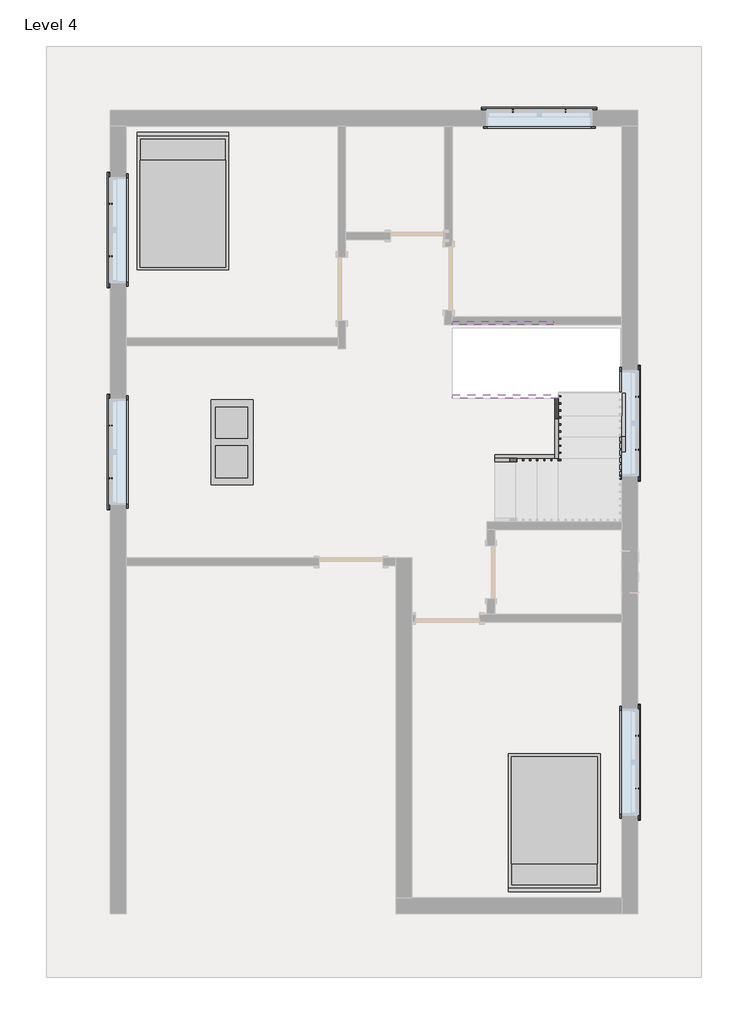
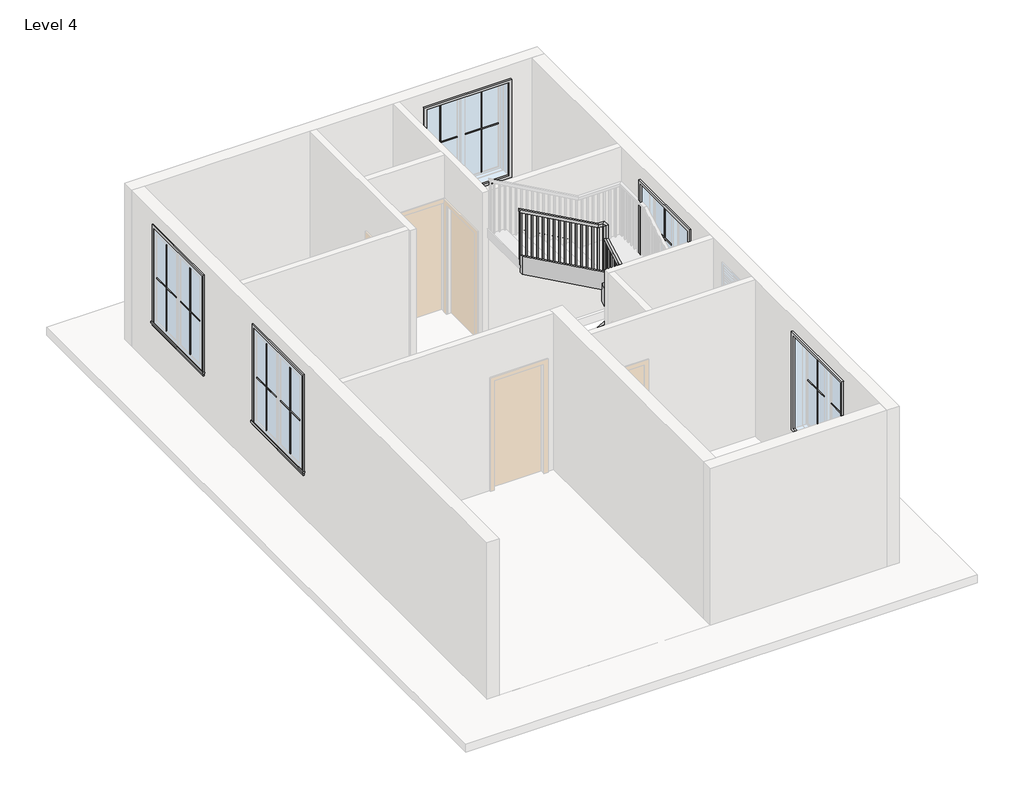
# One storey, part 2 of 2: 21 proxies, 6 members, 2 furniture elements, 1 railing.
"""IFC4 building model written with IfcOpenShell, lengths in millimetres."""

from ifc_helpers import new_model, si_unit, frame, origin, place, context, project, spatial, polyline, outline, extrude, faceted_brep, transform, mapped, element, save
from components import muntin_pattern_2x2_muntin_pattern_2x2_f6a80940, muntin_pattern_2x2_muntin_pattern_2x2_09b00a1c, trim_window_exterior_flat_with_sill_698ed857, trim_window_interior_flat_picture_frame_92551a5e, coffee_table_with_brass_mullions_11320_coffee_table_with_5962bef7, bed_17739_bed_17739_15c61121

model = new_model("IFC4")

# Units and contexts
model_context = context("Model", 3, world=origin())
ifc_project = project(units=[si_unit("LENGTHUNIT", "METRE", prefix="MILLI")], contexts=[model_context])

# Site, building, storey
site = spatial("IfcSite", under=ifc_project)
building = spatial("IfcBuilding", under=site)
storey = spatial("IfcBuildingStorey", under=building, Name="Level 4", Elevation=6400.8)

# Proxies
placement = place(None, origin())
muntin_pattern_2x2_muntin_pattern_2x2_shape = muntin_pattern_2x2_muntin_pattern_2x2_f6a80940(model_context)
element("IfcBuildingElementProxy", 1, Name="Muntin Pattern_2x2 : Muntin Pattern_2x2", ObjectType="Muntin Pattern_2x2 : Muntin Pattern_2x2", at=placement, inside=storey, context=model_context, shape_type="MappedRepresentation", body=[
    mapped(muntin_pattern_2x2_muntin_pattern_2x2_shape, transform((-4589.1575206, 441.8004493, 7385.05), x_axis=(0.0, 1.0, 0.0), y_axis=(-1.0, 0.0, 0.0), z_axis=(0.0, 0.0, 1.0))),
])
element("IfcBuildingElementProxy", 2, Name="Muntin Pattern_2x2 : Muntin Pattern_2x2", ObjectType="Muntin Pattern_2x2 : Muntin Pattern_2x2", at=placement, inside=storey, context=model_context, shape_type="MappedRepresentation", body=[
    mapped(muntin_pattern_2x2_muntin_pattern_2x2_shape, transform((-4589.1575206, 3632.6754493, 7385.05), x_axis=(0.0, 1.0, 0.0), y_axis=(-1.0, 0.0, 0.0), z_axis=(0.0, 0.0, 1.0))),
])
element("IfcBuildingElementProxy", 3, Name="Muntin Pattern_2x2 : Muntin Pattern_2x2", ObjectType="Muntin Pattern_2x2 : Muntin Pattern_2x2", at=placement, inside=storey, context=model_context, shape_type="MappedRepresentation", body=[
    mapped(muntin_pattern_2x2_muntin_pattern_2x2_shape, transform((1197.2799794, 5726.5879493, 7385.05), x_axis=(1.0, 0.0, 0.0), y_axis=(0.0, 1.0, 0.0), z_axis=(0.0, 0.0, 1.0))),
])
element("IfcBuildingElementProxy", 4, Name="Muntin Pattern_2x2 : Muntin Pattern_2x2", ObjectType="Muntin Pattern_2x2 : Muntin Pattern_2x2", at=placement, inside=storey, context=model_context, shape_type="MappedRepresentation", body=[
    mapped(muntin_pattern_2x2_muntin_pattern_2x2_shape, transform((2986.3924794, 1613.3754493, 7385.05), x_axis=(0.0, -1.0, 0.0), y_axis=(1.0, 0.0, 0.0), z_axis=(0.0, 0.0, 1.0))),
])
element("IfcBuildingElementProxy", 5, Name="Muntin Pattern_2x2 : Muntin Pattern_2x2", ObjectType="Muntin Pattern_2x2 : Muntin Pattern_2x2", at=placement, inside=storey, context=model_context, shape_type="MappedRepresentation", body=[
    mapped(muntin_pattern_2x2_muntin_pattern_2x2_shape, transform((2986.3924794, -3260.2495507, 7385.05), x_axis=(0.0, -1.0, 0.0), y_axis=(1.0, 0.0, 0.0), z_axis=(0.0, 0.0, 1.0))),
])
muntin_pattern_2x2_muntin_pattern_2x2_2_shape = muntin_pattern_2x2_muntin_pattern_2x2_09b00a1c(model_context)
element("IfcBuildingElementProxy", 6, Name="Muntin Pattern_2x2 : Muntin Pattern_2x2", ObjectType="Muntin Pattern_2x2 : Muntin Pattern_2x2", at=placement, inside=storey, context=model_context, shape_type="MappedRepresentation", body=[
    mapped(muntin_pattern_2x2_muntin_pattern_2x2_2_shape, transform((-4589.1575206, 1200.6254493, 7385.05), x_axis=(0.0, -1.0, 0.0), y_axis=(1.0, 0.0, 0.0), z_axis=(0.0, 0.0, 1.0))),
])
element("IfcBuildingElementProxy", 7, Name="Muntin Pattern_2x2 : Muntin Pattern_2x2", ObjectType="Muntin Pattern_2x2 : Muntin Pattern_2x2", at=placement, inside=storey, context=model_context, shape_type="MappedRepresentation", body=[
    mapped(muntin_pattern_2x2_muntin_pattern_2x2_2_shape, transform((-4589.1575206, 4391.5004493, 7385.05), x_axis=(0.0, -1.0, 0.0), y_axis=(1.0, 0.0, 0.0), z_axis=(0.0, 0.0, 1.0))),
])
element("IfcBuildingElementProxy", 8, Name="Muntin Pattern_2x2 : Muntin Pattern_2x2", ObjectType="Muntin Pattern_2x2 : Muntin Pattern_2x2", at=placement, inside=storey, context=model_context, shape_type="MappedRepresentation", body=[
    mapped(muntin_pattern_2x2_muntin_pattern_2x2_2_shape, transform((1956.1049794, 5726.5879493, 7385.05), x_axis=(-1.0, 0.0, 0.0), y_axis=(0.0, -1.0, 0.0), z_axis=(0.0, 0.0, 1.0))),
])
element("IfcBuildingElementProxy", 9, Name="Muntin Pattern_2x2 : Muntin Pattern_2x2", ObjectType="Muntin Pattern_2x2 : Muntin Pattern_2x2", at=placement, inside=storey, context=model_context, shape_type="MappedRepresentation", body=[
    mapped(muntin_pattern_2x2_muntin_pattern_2x2_2_shape, transform((2986.3924794, 854.5504493, 7385.05), x_axis=(0.0, 1.0, 0.0), y_axis=(-1.0, 0.0, 0.0), z_axis=(0.0, 0.0, 1.0))),
])
element("IfcBuildingElementProxy", 10, Name="Muntin Pattern_2x2 : Muntin Pattern_2x2", ObjectType="Muntin Pattern_2x2 : Muntin Pattern_2x2", at=placement, inside=storey, context=model_context, shape_type="MappedRepresentation", body=[
    mapped(muntin_pattern_2x2_muntin_pattern_2x2_2_shape, transform((2986.3924794, -4019.0745507, 7385.05), x_axis=(0.0, 1.0, 0.0), y_axis=(-1.0, 0.0, 0.0), z_axis=(0.0, 0.0, 1.0))),
])
trim_window_exterior_flat_with_sill_shape = trim_window_exterior_flat_with_sill_698ed857(model_context)
element("IfcBuildingElementProxy", 11, Name="Trim-Window-Exterior-Flat : with Sill", ObjectType="Trim-Window-Exterior-Flat : with Sill", at=placement, inside=storey, context=model_context, shape_type="MappedRepresentation", body=[
    mapped(trim_window_exterior_flat_with_sill_shape, transform((-4598.6825206, 821.2129493, 9144.0), x_axis=(0.0, -1.0, 0.0), y_axis=(0.0, 0.0, 1.0), z_axis=(-1.0, 0.0, 0.0))),
])
element("IfcBuildingElementProxy", 12, Name="Trim-Window-Exterior-Flat : with Sill", ObjectType="Trim-Window-Exterior-Flat : with Sill", at=placement, inside=storey, context=model_context, shape_type="MappedRepresentation", body=[
    mapped(trim_window_exterior_flat_with_sill_shape, transform((-4598.6825206, 4012.0879493, 9144.0), x_axis=(0.0, -1.0, 0.0), y_axis=(0.0, 0.0, 1.0), z_axis=(-1.0, 0.0, 0.0))),
])
element("IfcBuildingElementProxy", 13, Name="Trim-Window-Exterior-Flat : with Sill", ObjectType="Trim-Window-Exterior-Flat : with Sill", at=placement, inside=storey, context=model_context, shape_type="MappedRepresentation", body=[
    mapped(trim_window_exterior_flat_with_sill_shape, transform((1576.6924794, 5736.1129493, 9144.0), x_axis=(-1.0, 0.0, 0.0), y_axis=(0.0, 0.0, 1.0), z_axis=(0.0, 1.0, 0.0))),
])
element("IfcBuildingElementProxy", 14, Name="Trim-Window-Exterior-Flat : with Sill", ObjectType="Trim-Window-Exterior-Flat : with Sill", at=placement, inside=storey, context=model_context, shape_type="MappedRepresentation", body=[
    mapped(trim_window_exterior_flat_with_sill_shape, transform((2995.9174794, 1233.9629493, 9144.0), x_axis=(0.0, 1.0, 0.0), y_axis=(0.0, 0.0, 1.0), z_axis=(1.0, 0.0, 0.0))),
])
element("IfcBuildingElementProxy", 15, Name="Trim-Window-Exterior-Flat : with Sill", ObjectType="Trim-Window-Exterior-Flat : with Sill", at=placement, inside=storey, context=model_context, shape_type="MappedRepresentation", body=[
    mapped(trim_window_exterior_flat_with_sill_shape, transform((2995.9174794, -3639.6620507, 9144.0), x_axis=(0.0, 1.0, 0.0), y_axis=(0.0, 0.0, 1.0), z_axis=(1.0, 0.0, 0.0))),
])
trim_window_interior_flat_picture_frame_shape = trim_window_interior_flat_picture_frame_92551a5e(model_context)
element("IfcBuildingElementProxy", 16, Name="Trim-Window-Interior-Flat : Picture Frame", ObjectType="Trim-Window-Interior-Flat : Picture Frame", at=placement, inside=storey, context=model_context, shape_type="MappedRepresentation", body=[
    mapped(trim_window_interior_flat_picture_frame_shape, transform((-4370.0825206, 821.2129493, 9144.0), x_axis=(0.0, 1.0, 0.0), y_axis=(0.0, 0.0, 1.0), z_axis=(1.0, 0.0, 0.0))),
])
element("IfcBuildingElementProxy", 17, Name="Trim-Window-Interior-Flat : Picture Frame", ObjectType="Trim-Window-Interior-Flat : Picture Frame", at=placement, inside=storey, context=model_context, shape_type="MappedRepresentation", body=[
    mapped(trim_window_interior_flat_picture_frame_shape, transform((-4370.0825206, 4012.0879493, 9144.0), x_axis=(0.0, 1.0, 0.0), y_axis=(0.0, 0.0, 1.0), z_axis=(1.0, 0.0, 0.0))),
])
element("IfcBuildingElementProxy", 18, Name="Trim-Window-Interior-Flat : Picture Frame", ObjectType="Trim-Window-Interior-Flat : Picture Frame", at=placement, inside=storey, context=model_context, shape_type="MappedRepresentation", body=[
    mapped(trim_window_interior_flat_picture_frame_shape, transform((1576.6924794, 5507.5129493, 9144.0), x_axis=(1.0, 0.0, 0.0), y_axis=(0.0, 0.0, 1.0), z_axis=(0.0, -1.0, 0.0))),
])
element("IfcBuildingElementProxy", 19, Name="Trim-Window-Interior-Flat : Picture Frame", ObjectType="Trim-Window-Interior-Flat : Picture Frame", at=placement, inside=storey, context=model_context, shape_type="MappedRepresentation", body=[
    mapped(trim_window_interior_flat_picture_frame_shape, transform((2767.3174794, 1233.9629493, 9144.0), x_axis=(0.0, -1.0, 0.0), y_axis=(0.0, 0.0, 1.0), z_axis=(-1.0, 0.0, 0.0))),
])
element("IfcBuildingElementProxy", 20, Name="Trim-Window-Interior-Flat : Picture Frame", ObjectType="Trim-Window-Interior-Flat : Picture Frame", at=placement, inside=storey, context=model_context, shape_type="MappedRepresentation", body=[
    mapped(trim_window_interior_flat_picture_frame_shape, transform((2767.3174794, -3639.6620507, 9144.0), x_axis=(0.0, -1.0, 0.0), y_axis=(0.0, 0.0, 1.0), z_axis=(-1.0, 0.0, 0.0))),
])
coffee_table_with_brass_mullions_11320_coffee_table_with_shape = coffee_table_with_brass_mullions_11320_coffee_table_with_5962bef7(model_context)
element("IfcBuildingElementProxy", 21, Name="coffee_table_with_brass_mullions_11320 : coffee_table_with_brass_mullions_11320", ObjectType="coffee_table_with_brass_mullions_11320 : coffee_table_with_brass_mullions_11320", at=placement, inside=storey, context=model_context, shape_type="MappedRepresentation", body=[
    mapped(coffee_table_with_brass_mullions_11320_coffee_table_with_shape, transform((-2412.0418112, 1596.9678033, 6400.8), x_axis=(0.0, 1.0, 0.0), y_axis=(-1.0, 0.0, 0.0), z_axis=(0.0, 0.0, 1.0))),
])

# Furniture
bed_17739_bed_17739_shape = bed_17739_bed_17739_15c61121(model_context)
element("IfcFurniture", 22, ObjectType="Bed_17739 : Bed_17739", at=placement, inside=storey, context=model_context, shape_type="MappedRepresentation", body=[
    mapped(bed_17739_bed_17739_shape, transform((-3550.9325206, 4402.6129493, 6400.8), x_axis=(1.0, 0.0, 0.0), y_axis=(0.0, 1.0, 0.0), z_axis=(0.0, 0.0, 1.0))),
])
element("IfcFurniture", 23, ObjectType="Bed_17739 : Bed_17739", at=placement, inside=storey, context=model_context, shape_type="MappedRepresentation", body=[
    mapped(bed_17739_bed_17739_shape, transform((1795.7674794, -4487.3870507, 6400.8), x_axis=(-1.0, 0.0, 0.0), y_axis=(0.0, -1.0, 0.0), z_axis=(0.0, 0.0, 1.0))),
])

# Members
element("IfcMember", 24, ObjectType="Stringer - 2\" Width", at=placement, inside=storey, context=model_context, shape_type="SweptSolid", body=[
    extrude(outline(polyline([(6608.3983948, 938.5174794), (6400.8, 938.5174794), (6400.8, 1192.4619822), (6739.4974984, 1802.1174794), (7088.1761726, 1802.1174794), (6608.3983948, 938.5174794)])), frame((0.0, 732.3129493, 0.0), z_axis=(0.0, 1.0, 0.0), x_axis=(0.0, 0.0, 1.0)), (0.0, 0.0, 1.0), 50.8),
])
element("IfcMember", 25, ObjectType="Stringer - 2\" Width", at=placement, inside=storey, context=model_context, shape_type="SweptSolid", body=[
    extrude(outline(polyline([(732.3129493, 6937.053054), (732.3129493, 7285.7317281), (1595.9129493, 7765.5095059), (1595.9129493, 7416.8308318), (732.3129493, 6937.053054)])), frame((1802.1174794, 0.0, 0.0), z_axis=(1.0, 0.0, 0.0), x_axis=(0.0, 1.0, 0.0)), (0.0, 0.0, 1.0), 50.8),
])
element("IfcMember", 26, ObjectType="Stringer - 2\" Width", at=placement, inside=storey, context=model_context, shape_type="SweptSolid", body=[
    extrude(outline(polyline([(7614.3863873, 1852.9174794), (7963.0650614, 1852.9174794), (8809.7317281, 328.9174794), (8461.053054, 328.9174794), (7614.3863873, 1852.9174794)])), frame((0.0, 1595.9129493, 0.0), z_axis=(0.0, 1.0, 0.0), x_axis=(0.0, 0.0, 1.0)), (0.0, 0.0, 1.0), 50.8),
])
element("IfcMember", 27, ObjectType="Stringer - 2\" Width", at=placement, inside=storey, context=model_context, shape_type="SweptSolid", body=[
    extrude(outline(polyline([(6608.3983948, 938.5174794), (6400.8, 938.5174794), (6400.8, 1192.4619822), (6777.7317281, 1870.9390928), (6777.7317281, 1243.3174794), (6608.3983948, 938.5174794)])), frame((0.0, -232.8870507, 0.0), z_axis=(0.0, 1.0, 0.0), x_axis=(0.0, 0.0, 1.0)), (0.0, 0.0, 1.0), 50.8),
])
element("IfcMember", 28, ObjectType="Stringer - 2\" Width", at=placement, inside=storey, context=model_context, shape_type="SweptSolid", body=[
    extrude(outline(polyline([(714.2913359, 7275.7197207), (1037.1129493, 7455.0650614), (1664.7345627, 7455.0650614), (1341.9129493, 7275.7197207), (714.2913359, 7275.7197207)])), frame((2767.3174794, 0.0, 0.0), z_axis=(1.0, 0.0, 0.0), x_axis=(0.0, 1.0, 0.0)), (0.0, 0.0, 1.0), 50.8),
])
element("IfcMember", 29, ObjectType="Stringer - 2\" Width", at=placement, inside=storey, context=model_context, shape_type="SweptSolid", body=[
    extrude(outline(polyline([(8002.4419429, 1782.0390928), (8809.7317281, 328.9174794), (8461.053054, 328.9174794), (8002.4419429, 1154.4174794), (8002.4419429, 1782.0390928)])), frame((0.0, 2650.0129493, 0.0), z_axis=(0.0, 1.0, 0.0), x_axis=(0.0, 0.0, 1.0)), (0.0, 0.0, 1.0), 50.8),
])

# Railing
element("IfcRailing", 30, ObjectType="Handrail - Rectangular", at=placement, inside=storey, context=model_context, shape_type="SolidModel", body=[
    faceted_brep([(938.5174794, 732.3129493, 7484.5333333), (938.5174794, 732.3129493, 7426.420221), (938.5174794, 681.5129493, 7426.420221), (938.5174794, 681.5129493, 7484.5333333), (1776.7174794, 732.3129493, 7950.2), (1827.5174794, 732.3129493, 7920.3091099), (1827.5174794, 681.5129493, 7920.3091099), (1776.7174794, 681.5129493, 7950.2), (1776.7174794, 732.3129493, 8204.2), (1827.5174794, 732.3129493, 8153.4), (1827.5174794, 681.5129493, 8153.4), (1776.7174794, 681.5129493, 8204.2), (1852.9174794, 732.3129493, 8204.2), (1852.9174794, 732.3129493, 8153.4), (1903.7174794, 681.5129493, 8153.4), (1903.7174794, 681.5129493, 8204.2), (1852.9174794, 808.5129493, 8204.2), (1852.9174794, 821.6765516, 8153.4), (1903.7174794, 821.6765516, 8153.4), (1903.7174794, 808.5129493, 8204.2), (1852.9174794, 1570.5129493, 8627.5333333), (1852.9174794, 1621.3129493, 8597.6424432), (1903.7174794, 1621.3129493, 8597.6424432), (1903.7174794, 1570.5129493, 8627.5333333), (1852.9174794, 1570.5129493, 8881.5333333), (1852.9174794, 1621.3129493, 8830.7333333), (1903.7174794, 1621.3129493, 8830.7333333), (1903.7174794, 1570.5129493, 8881.5333333), (1852.9174794, 1646.7129493, 8881.5333333), (1852.9174794, 1646.7129493, 8830.7333333), (1903.7174794, 1697.5129493, 8830.7333333), (1903.7174794, 1697.5129493, 8881.5333333), (1776.7174794, 1646.7129493, 8881.5333333), (1763.5538772, 1646.7129493, 8830.7333333), (1763.5538772, 1697.5129493, 8830.7333333), (1776.7174794, 1697.5129493, 8881.5333333), (328.9174794, 1646.7129493, 9685.8666667), (328.9174794, 1697.5129493, 9685.8666667), (328.9174794, 1697.5129493, 9627.7535543), (328.9174794, 1646.7129493, 9627.7535543)], [[[0, 1, 2, 3]], [[1, 0, 4, 5]], [[2, 1, 5, 6]], [[3, 2, 6, 7]], [[0, 3, 7, 4]], [[5, 4, 8, 9]], [[6, 5, 9, 10]], [[7, 6, 10, 11]], [[4, 7, 11, 8]], [[9, 8, 12, 13]], [[10, 9, 13, 14]], [[11, 10, 14, 15]], [[8, 11, 15, 12]], [[13, 12, 16, 17]], [[14, 13, 17, 18]], [[15, 14, 18, 19]], [[12, 15, 19, 16]], [[17, 16, 20, 21]], [[18, 17, 21, 22]], [[19, 18, 22, 23]], [[16, 19, 23, 20]], [[21, 20, 24, 25]], [[22, 21, 25, 26]], [[23, 22, 26, 27]], [[20, 23, 27, 24]], [[25, 24, 28, 29]], [[26, 25, 29, 30]], [[27, 26, 30, 31]], [[24, 27, 31, 28]], [[29, 28, 32, 33]], [[30, 29, 33, 34]], [[31, 30, 34, 35]], [[28, 31, 35, 32]], [[36, 37, 38, 39]], [[33, 32, 36, 39]], [[34, 33, 39, 38]], [[35, 34, 38, 37]], [[32, 35, 37, 36]]]),
    extrude(outline(polyline([(9618.9341099, 344.7924794), (8602.1333333, 344.7924794), (8602.1333333, 363.8424794), (9608.3507765, 363.8424794), (9618.9341099, 344.7924794)])), frame((0.0, 1662.5879493, 0.0), z_axis=(0.0, 1.0, 0.0), x_axis=(0.0, 0.0, 1.0)), (0.0, 0.0, 1.0), 19.05),
    extrude(outline(polyline([(9562.4896654, 446.3924794), (8602.1333333, 446.3924794), (8602.1333333, 465.4424794), (9551.9063321, 465.4424794), (9562.4896654, 446.3924794)])), frame((0.0, 1662.5879493, 0.0), z_axis=(0.0, 1.0, 0.0), x_axis=(0.0, 0.0, 1.0)), (0.0, 0.0, 1.0), 19.05),
    extrude(outline(polyline([(9506.045221, 547.9924794), (8602.1333333, 547.9924794), (8602.1333333, 567.0424794), (9495.4618876, 567.0424794), (9506.045221, 547.9924794)])), frame((0.0, 1662.5879493, 0.0), z_axis=(0.0, 1.0, 0.0), x_axis=(0.0, 0.0, 1.0)), (0.0, 0.0, 1.0), 19.05),
    extrude(outline(polyline([(9449.6007765, 649.5924794), (8432.8, 649.5924794), (8432.8, 668.6424794), (9439.0174432, 668.6424794), (9449.6007765, 649.5924794)])), frame((0.0, 1662.5879493, 0.0), z_axis=(0.0, 1.0, 0.0), x_axis=(0.0, 0.0, 1.0)), (0.0, 0.0, 1.0), 19.05),
    extrude(outline(polyline([(9393.1563321, 751.1924794), (8432.8, 751.1924794), (8432.8, 770.2424794), (9382.5729988, 770.2424794), (9393.1563321, 751.1924794)])), frame((0.0, 1662.5879493, 0.0), z_axis=(0.0, 1.0, 0.0), x_axis=(0.0, 0.0, 1.0)), (0.0, 0.0, 1.0), 19.05),
    extrude(outline(polyline([(9336.7118876, 852.7924794), (8432.8, 852.7924794), (8432.8, 871.8424794), (9326.1285543, 871.8424794), (9336.7118876, 852.7924794)])), frame((0.0, 1662.5879493, 0.0), z_axis=(0.0, 1.0, 0.0), x_axis=(0.0, 0.0, 1.0)), (0.0, 0.0, 1.0), 19.05),
    extrude(outline(polyline([(9280.2674432, 954.3924794), (8263.4666667, 954.3924794), (8263.4666667, 973.4424794), (9269.6841099, 973.4424794), (9280.2674432, 954.3924794)])), frame((0.0, 1662.5879493, 0.0), z_axis=(0.0, 1.0, 0.0), x_axis=(0.0, 0.0, 1.0)), (0.0, 0.0, 1.0), 19.05),
    extrude(outline(polyline([(9223.8229988, 1055.9924794), (8263.4666667, 1055.9924794), (8263.4666667, 1075.0424794), (9213.2396654, 1075.0424794), (9223.8229988, 1055.9924794)])), frame((0.0, 1662.5879493, 0.0), z_axis=(0.0, 1.0, 0.0), x_axis=(0.0, 0.0, 1.0)), (0.0, 0.0, 1.0), 19.05),
    extrude(outline(polyline([(9167.3785543, 1157.5924794), (8263.4666667, 1157.5924794), (8263.4666667, 1176.6424794), (9156.795221, 1176.6424794), (9167.3785543, 1157.5924794)])), frame((0.0, 1662.5879493, 0.0), z_axis=(0.0, 1.0, 0.0), x_axis=(0.0, 0.0, 1.0)), (0.0, 0.0, 1.0), 19.05),
    extrude(outline(polyline([(9110.9341099, 1259.1924794), (8094.1333333, 1259.1924794), (8094.1333333, 1278.2424794), (9100.3507765, 1278.2424794), (9110.9341099, 1259.1924794)])), frame((0.0, 1662.5879493, 0.0), z_axis=(0.0, 1.0, 0.0), x_axis=(0.0, 0.0, 1.0)), (0.0, 0.0, 1.0), 19.05),
    extrude(outline(polyline([(9054.4896654, 1360.7924794), (8094.1333333, 1360.7924794), (8094.1333333, 1379.8424794), (9043.9063321, 1379.8424794), (9054.4896654, 1360.7924794)])), frame((0.0, 1662.5879493, 0.0), z_axis=(0.0, 1.0, 0.0), x_axis=(0.0, 0.0, 1.0)), (0.0, 0.0, 1.0), 19.05),
    extrude(outline(polyline([(8998.045221, 1462.3924794), (8094.1333333, 1462.3924794), (8094.1333333, 1481.4424794), (8987.4618876, 1481.4424794), (8998.045221, 1462.3924794)])), frame((0.0, 1662.5879493, 0.0), z_axis=(0.0, 1.0, 0.0), x_axis=(0.0, 0.0, 1.0)), (0.0, 0.0, 1.0), 19.05),
    extrude(outline(polyline([(8941.6007765, 1563.9924794), (7924.8, 1563.9924794), (7924.8, 1583.0424794), (8931.0174432, 1583.0424794), (8941.6007765, 1563.9924794)])), frame((0.0, 1662.5879493, 0.0), z_axis=(0.0, 1.0, 0.0), x_axis=(0.0, 0.0, 1.0)), (0.0, 0.0, 1.0), 19.05),
    extrude(outline(polyline([(8885.1563321, 1665.5924794), (7924.8, 1665.5924794), (7924.8, 1684.6424794), (8874.5729988, 1684.6424794), (8885.1563321, 1665.5924794)])), frame((0.0, 1662.5879493, 0.0), z_axis=(0.0, 1.0, 0.0), x_axis=(0.0, 0.0, 1.0)), (0.0, 0.0, 1.0), 19.05),
    extrude(outline(polyline([(8828.7118876, 1767.1924794), (7924.8, 1767.1924794), (7924.8, 1786.2424794), (8818.1285543, 1786.2424794), (8828.7118876, 1767.1924794)])), frame((0.0, 1662.5879493, 0.0), z_axis=(0.0, 1.0, 0.0), x_axis=(0.0, 0.0, 1.0)), (0.0, 0.0, 1.0), 19.05),
    extrude(outline(polyline([(1868.7924794, 1611.7879493), (1868.7924794, 1630.8379493), (1887.8424794, 1630.8379493), (1887.8424794, 1611.7879493), (1868.7924794, 1611.7879493)])), frame((0.0, 0.0, 7586.1333333), z_axis=(0.0, 0.0, 1.0), x_axis=(1.0, 0.0, 0.0)), (0.0, 0.0, 1.0), 1244.6),
    extrude(outline(polyline([(1529.2379493, 8546.4896654), (1529.2379493, 7586.1333333), (1510.1879493, 7586.1333333), (1510.1879493, 8535.9063321), (1529.2379493, 8546.4896654)])), frame((1868.7924794, 0.0, 0.0), z_axis=(1.0, 0.0, 0.0), x_axis=(0.0, 1.0, 0.0)), (0.0, 0.0, 1.0), 19.05),
    extrude(outline(polyline([(1427.6379493, 8490.045221), (1427.6379493, 7586.1333333), (1408.5879493, 7586.1333333), (1408.5879493, 8479.4618876), (1427.6379493, 8490.045221)])), frame((1868.7924794, 0.0, 0.0), z_axis=(1.0, 0.0, 0.0), x_axis=(0.0, 1.0, 0.0)), (0.0, 0.0, 1.0), 19.05),
    extrude(outline(polyline([(1326.0379493, 8433.6007765), (1326.0379493, 7416.8), (1306.9879493, 7416.8), (1306.9879493, 8423.0174432), (1326.0379493, 8433.6007765)])), frame((1868.7924794, 0.0, 0.0), z_axis=(1.0, 0.0, 0.0), x_axis=(0.0, 1.0, 0.0)), (0.0, 0.0, 1.0), 19.05),
    extrude(outline(polyline([(1224.4379493, 8377.1563321), (1224.4379493, 7416.8), (1205.3879493, 7416.8), (1205.3879493, 8366.5729988), (1224.4379493, 8377.1563321)])), frame((1868.7924794, 0.0, 0.0), z_axis=(1.0, 0.0, 0.0), x_axis=(0.0, 1.0, 0.0)), (0.0, 0.0, 1.0), 19.05),
    extrude(outline(polyline([(1122.8379493, 8320.7118876), (1122.8379493, 7416.8), (1103.7879493, 7416.8), (1103.7879493, 8310.1285543), (1122.8379493, 8320.7118876)])), frame((1868.7924794, 0.0, 0.0), z_axis=(1.0, 0.0, 0.0), x_axis=(0.0, 1.0, 0.0)), (0.0, 0.0, 1.0), 19.05),
    extrude(outline(polyline([(1021.2379493, 8264.2674432), (1021.2379493, 7247.4666667), (1002.1879493, 7247.4666667), (1002.1879493, 8253.6841099), (1021.2379493, 8264.2674432)])), frame((1868.7924794, 0.0, 0.0), z_axis=(1.0, 0.0, 0.0), x_axis=(0.0, 1.0, 0.0)), (0.0, 0.0, 1.0), 19.05),
    extrude(outline(polyline([(919.6379493, 8207.8229988), (919.6379493, 7247.4666667), (900.5879493, 7247.4666667), (900.5879493, 8197.2396654), (919.6379493, 8207.8229988)])), frame((1868.7924794, 0.0, 0.0), z_axis=(1.0, 0.0, 0.0), x_axis=(0.0, 1.0, 0.0)), (0.0, 0.0, 1.0), 19.05),
    extrude(outline(polyline([(818.0379493, 8151.3785543), (818.0379493, 7247.4666667), (798.9879493, 7247.4666667), (798.9879493, 8140.795221), (818.0379493, 8151.3785543)])), frame((1868.7924794, 0.0, 0.0), z_axis=(1.0, 0.0, 0.0), x_axis=(0.0, 1.0, 0.0)), (0.0, 0.0, 1.0), 19.05),
    extrude(outline(polyline([(1843.3924794, 716.4379493), (1862.4424794, 716.4379493), (1862.4424794, 697.3879493), (1843.3924794, 697.3879493), (1843.3924794, 716.4379493)])), frame((0.0, 0.0, 7078.1333333), z_axis=(0.0, 0.0, 1.0), x_axis=(1.0, 0.0, 0.0)), (0.0, 0.0, 1.0), 1075.2666667),
    extrude(outline(polyline([(7872.6841099, 1741.7924794), (6908.8, 1741.7924794), (6908.8, 1760.8424794), (7883.2674432, 1760.8424794), (7872.6841099, 1741.7924794)])), frame((0.0, 697.3879493, 0.0), z_axis=(0.0, 1.0, 0.0), x_axis=(0.0, 0.0, 1.0)), (0.0, 0.0, 1.0), 19.05),
    extrude(outline(polyline([(7816.2396654, 1640.1924794), (6908.8, 1640.1924794), (6908.8, 1659.2424794), (7826.8229988, 1659.2424794), (7816.2396654, 1640.1924794)])), frame((0.0, 697.3879493, 0.0), z_axis=(0.0, 1.0, 0.0), x_axis=(0.0, 0.0, 1.0)), (0.0, 0.0, 1.0), 19.05),
    extrude(outline(polyline([(7759.795221, 1538.5924794), (6908.8, 1538.5924794), (6908.8, 1557.6424794), (7770.3785543, 1557.6424794), (7759.795221, 1538.5924794)])), frame((0.0, 697.3879493, 0.0), z_axis=(0.0, 1.0, 0.0), x_axis=(0.0, 0.0, 1.0)), (0.0, 0.0, 1.0), 19.05),
    extrude(outline(polyline([(7703.3507765, 1436.9924794), (6739.4666667, 1436.9924794), (6739.4666667, 1456.0424794), (7713.9341099, 1456.0424794), (7703.3507765, 1436.9924794)])), frame((0.0, 697.3879493, 0.0), z_axis=(0.0, 1.0, 0.0), x_axis=(0.0, 0.0, 1.0)), (0.0, 0.0, 1.0), 19.05),
    extrude(outline(polyline([(7646.9063321, 1335.3924794), (6739.4666667, 1335.3924794), (6739.4666667, 1354.4424794), (7657.4896654, 1354.4424794), (7646.9063321, 1335.3924794)])), frame((0.0, 697.3879493, 0.0), z_axis=(0.0, 1.0, 0.0), x_axis=(0.0, 0.0, 1.0)), (0.0, 0.0, 1.0), 19.05),
    extrude(outline(polyline([(7590.4618876, 1233.7924794), (6739.4666667, 1233.7924794), (6739.4666667, 1252.8424794), (7601.045221, 1252.8424794), (7590.4618876, 1233.7924794)])), frame((0.0, 697.3879493, 0.0), z_axis=(0.0, 1.0, 0.0), x_axis=(0.0, 0.0, 1.0)), (0.0, 0.0, 1.0), 19.05),
    extrude(outline(polyline([(7534.0174432, 1132.1924794), (6570.1333333, 1132.1924794), (6570.1333333, 1151.2424794), (7544.6007765, 1151.2424794), (7534.0174432, 1132.1924794)])), frame((0.0, 697.3879493, 0.0), z_axis=(0.0, 1.0, 0.0), x_axis=(0.0, 0.0, 1.0)), (0.0, 0.0, 1.0), 19.05),
    extrude(outline(polyline([(7477.5729988, 1030.5924794), (6570.1333333, 1030.5924794), (6570.1333333, 1049.6424794), (7488.1563321, 1049.6424794), (7477.5729988, 1030.5924794)])), frame((0.0, 697.3879493, 0.0), z_axis=(0.0, 1.0, 0.0), x_axis=(0.0, 0.0, 1.0)), (0.0, 0.0, 1.0), 19.05),
    extrude(outline(polyline([(1868.7924794, 1662.5879493), (1868.7924794, 1681.6379493), (1887.8424794, 1681.6379493), (1887.8424794, 1662.5879493), (1868.7924794, 1662.5879493)])), frame((0.0, 0.0, 7755.4666667), z_axis=(0.0, 0.0, 1.0), x_axis=(1.0, 0.0, 0.0)), (0.0, 0.0, 1.0), 1075.2666667),
    extrude(outline(polyline([(1868.7924794, 716.4379493), (1887.8424794, 716.4379493), (1887.8424794, 697.3879493), (1868.7924794, 697.3879493), (1868.7924794, 716.4379493)])), frame((0.0, 0.0, 7078.1333333), z_axis=(0.0, 0.0, 1.0), x_axis=(1.0, 0.0, 0.0)), (0.0, 0.0, 1.0), 1075.2666667),
    extrude(outline(polyline([(9627.7535543, 328.9174794), (8602.1333333, 328.9174794), (8602.1333333, 347.9674794), (9617.170221, 347.9674794), (9627.7535543, 328.9174794)])), frame((0.0, 1662.5879493, 0.0), z_axis=(0.0, 1.0, 0.0), x_axis=(0.0, 0.0, 1.0)), (0.0, 0.0, 1.0), 19.05),
    extrude(outline(polyline([(7426.420221, 938.5174794), (6570.1333333, 938.5174794), (6570.1333333, 957.5674794), (7437.0035543, 957.5674794), (7426.420221, 938.5174794)])), frame((0.0, 697.3879493, 0.0), z_axis=(0.0, 1.0, 0.0), x_axis=(0.0, 0.0, 1.0)), (0.0, 0.0, 1.0), 19.05),
])

save(model, "model.ifc")

# Revit data of these elements
# Type "Muntin Pattern_2x2 : Muntin Pattern_2x2"
#   Width [instance default] = 4' - 0"
#   Thickness = 0' - 0 1/2"
#   Height [instance default] = 4' - 0"
#   Distance = 0' - 0 3/4"
#   Interior Material [instance default] = none
#   Exterior Material [instance default] = none
#   Default Elevation = 0
# Type "Trim-Window-Exterior-Flat : with Sill"
#   Trim Width = 0' - 2 1/4"
#   Trim Thickness_Picture Frame = 0' - 1 1/4"
#   Trim Thickness_with Sill = 0' - 0 3/4"
#   Sill Thickness = 0' - 1 1/4"
#   Opening Width [instance default] = 2' - 0"
#   Opening Height [instance default] = 3' - 0"
#   Default Elevation = 4' - 0"
#   Sill = yes
#   Picture Frame = no
#   Trim Material [instance default] = none
# Type "Trim-Window-Interior-Flat : Picture Frame"
#   Trim Thickness_Picture Frame = 0' - 1 1/4"
#   Trim Width = 0' - 2 1/4"
#   Trim Thickness_with Sill = 0' - 0 3/4"
#   Sill Thickness = 0' - 1 1/4"
#   Opening Width [instance default] = 2' - 0"
#   Opening Height [instance default] = 3' - 0"
#   Default Elevation = 4' - 0"
#   Sill = no
#   Picture Frame = yes
#   Trim Material [instance default] = none
# Type "coffee_table_with_brass_mullions_11320 : coffee_table_with_brass_mullions_11320"
#   Default Elevation = 0
# Type "Bed_17739 : Bed_17739"
#   Default Elevation = 0
# Type "Handrail - Rectangular"
#   Assembly Code = "C2010400"
#   built-in parameter 1008612 = 0.0416667 (stored number, unit not read)
#   built-in parameter 1008611 = 0.0416667 (stored number, unit not read)
#   built-in parameter 1008609 = 0.333333 (stored number, unit not read)
#   built-in parameter 1008604 = 0.166667 (stored number, unit not read)
#   built-in parameter 1008603 = 0.166667 (stored number, unit not read)
#   Railing Height = 3' - 0"
#   built-in parameter 1008630 = 2
#   built-in parameter 1008610 = 2
#   built-in parameter 1008618 = Baluster - Square : 3/4"
# Elements 1, 2, 3, 4, 5, 6, 7, 8, 9, 10 (IfcBuildingElementProxy, "Muntin Pattern_2x2 : Muntin Pattern_2x2")
#   Width = 2' - 0 5/8"
#   Height = 5' - 6 1/2"
#   Interior Material = Wood - Stained
#   Exterior Material = Clad - White
#   Phase Created = New Construction
#   Materials on its faces: "Clad - White", "Wood - Stained"
# Elements 11, 12, 13, 14, 15 (IfcBuildingElementProxy, "Trim-Window-Exterior-Flat : with Sill")
#   Opening Width = 5' - 0"
#   Opening Height = 6' - 0"
#   Trim Material = Clad - White
#   Phase Created = New Construction
#   Materials on its faces: "Clad - White"
# Elements 16, 17, 18, 19, 20 (IfcBuildingElementProxy, "Trim-Window-Interior-Flat : Picture Frame")
#   Opening Width = 5' - 0"
#   Opening Height = 6' - 0"
#   Trim Material = Wood - Stained
#   Phase Created = New Construction
#   Materials on its faces: "Wood - Stained"
# Element 21 (IfcBuildingElementProxy, "coffee_table_with_brass_mullions_11320 : coffee_table_with_brass_mullions_11320")
#   Phase Created = New Construction
#   Materials on its faces: "Default Wall", "TABLE", "Glass", "Default"
# Elements 22, 23 (IfcFurniture, "Bed_17739 : Bed_17739")
#   Phase Created = New Construction
#   Materials on its faces: "legs", "sheets", "bed frame", "Blanket"
# Elements 24, 25, 26, 27, 28, 29 (IfcMember, "Stringer - 2\" Width")
#   Phase Created = New Construction
# Element 30 (IfcRailing, "Handrail - Rectangular")
#   Phase Created = New Construction
# Materials
#   "Clad - White": class "Wood", colour RGB 242 242 238, transparency 0, Cost = 0
#   "Wood - Stained": class "Wood", colour RGB 224 178 126, transparency 0, Cost = 0
#   "Default Wall": colour RGB 128 128 128, transparency 0, Cost = 0
#   "TABLE": class "Generic", colour RGB 120 120 120, transparency 0, Cost = 0
#   "Glass": class "Glass", colour RGB 0 128 192, transparency 0.75, Description = "Soda Lime Glass", Cost = 0
#   "Default": colour RGB 127 127 127, transparency 0, Cost = 0
#   "legs": colour RGB 90 73 37, transparency 0, Cost = 0
#   "sheets": colour RGB 200 195 176, transparency 0, Cost = 0
#   "bed frame": colour RGB 90 73 37, transparency 0, Cost = 0
#   "Blanket": class "System", colour RGB 59 0 1, transparency 0, Cost = 0
